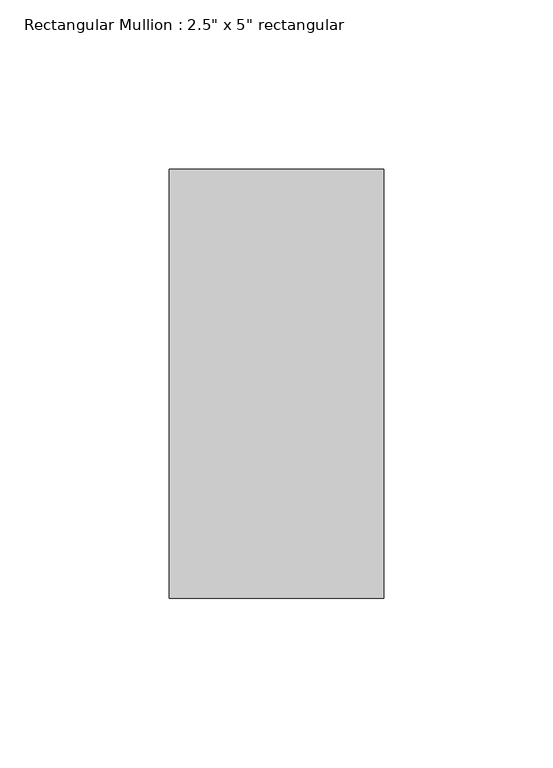
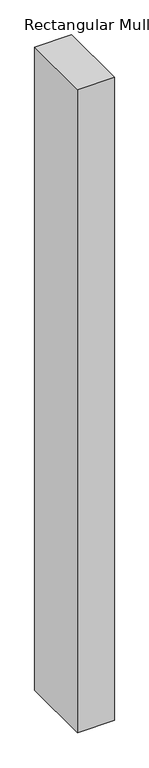
"""IFC4 building model written with IfcOpenShell, lengths in millimetres: member geometry."""

from ifc_helpers import new_model, si_unit, frame, origin, place, context, project, spatial, polyline, outline, extrude, source, transform, mapped, element, save


def member_e9460d8e(model_context):
    return source(origin(), model_context, "Body", "SweptSolid", [
        extrude(outline(polyline([(31.75, 63.5), (31.75, -63.5), (-31.75, -63.5), (-31.75, 63.5), (31.75, 63.5)])), frame((0.0, 0.0, -1168.4), z_axis=(0.0, 0.0, 1.0), x_axis=(1.0, 0.0, 0.0)), (0.0, 0.0, 1.0), 1168.4),
    ])


if __name__ == "__main__":
    model = new_model("IFC4")
    model_context = context("Model", 3, world=origin())
    ifc_project = project(units=[si_unit("LENGTHUNIT", "METRE", prefix="MILLI")], contexts=[model_context])
    site = spatial("IfcSite", under=ifc_project)
    building = spatial("IfcBuilding", under=site)
    placement = place(None, origin())
    member_shape = member_e9460d8e(model_context)
    element("IfcMember", 1, ObjectType="Rectangular Mullion : 2.5\" x 5\" rectangular", at=placement, inside=building, context=model_context, shape_type="MappedRepresentation", body=[
        mapped(member_shape, transform((0.0, 0.0, 0.0), x_axis=(1.0, 0.0, 0.0), y_axis=(0.0, 1.0, 0.0), z_axis=(0.0, 0.0, 1.0))),
    ])
    save(model, "model.ifc")

# Revit data of these elements
# Type "Rectangular Mullion : 2.5\" x 5\" rectangular"
#   built-in parameter 1007304 = 0.416667 (stored number, unit not read)
#   built-in parameter 1007301 = 0.104167 (stored number, unit not read)
#   built-in parameter 1007300 = 0.104167 (stored number, unit not read)
# Element 1 (IfcMember, "Rectangular Mullion : 2.5\" x 5\" rectangular")
#   Materials on its faces: "Roofing, EPDM Membrane"
# Materials
#   "Roofing, EPDM Membrane": class "Generic", colour RGB 127 127 127, transparency 0, Description = "EPDM roof membrane", Cost = 0
